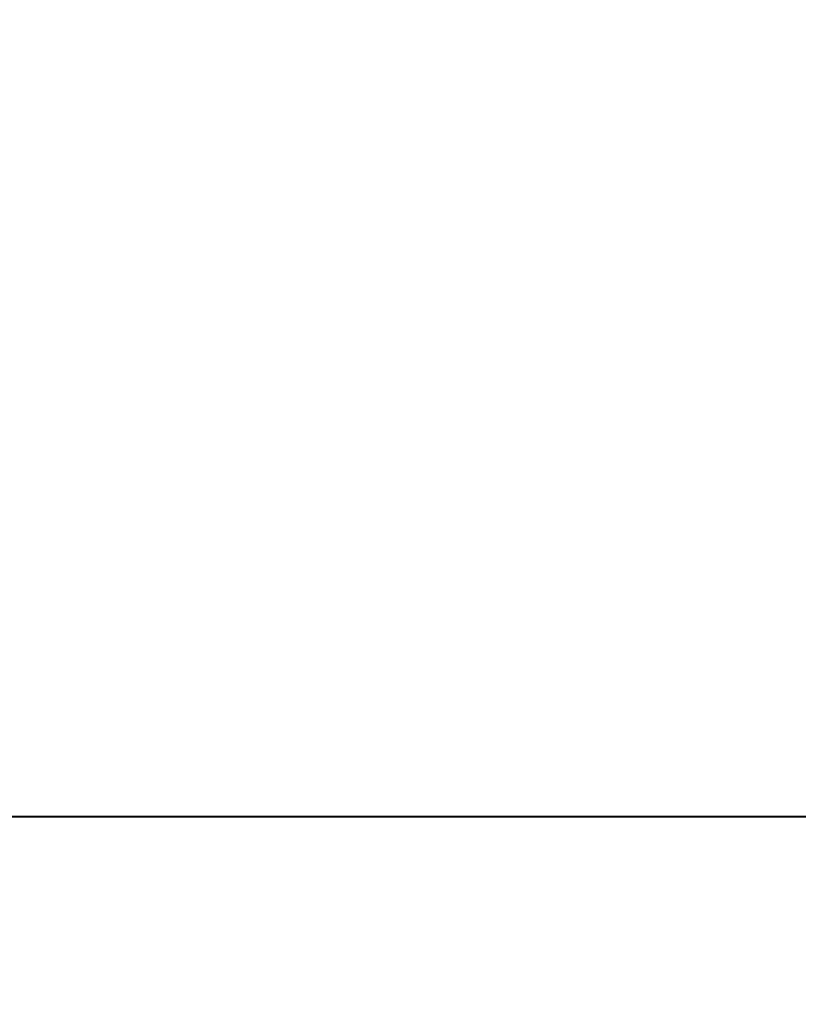
# Model space of a CAD drawing. Units: inches. Extents: x 459864 to 460310, y 324185 to 324787.
# Tile 80 of 112: x 460238.11 to 460246.61, y 324281.44 to 324292.19. Entities that reach past the tile are written whole.
import ezdxf

# ---------------------------------------------------------------- set-up
doc = ezdxf.new("R2010")
doc.units = ezdxf.units.IN
for name, color, linetype, lineweight in [('A-ANNO-DIMS', 2, 'Continuous', 18), ('A-WALL', 7, 'Continuous', 40), ('L-SITE-PATT', 252, 'Continuous', 13)]:
    doc.layers.add(name, color=color, linetype=linetype, lineweight=lineweight)
doc.styles.get("Standard").update_dxf_attribs({"font": 'arial.ttf'})
doc.dimstyles.new('ISO-25', dxfattribs={"dimtxt": 6, "dimasz": 2.5, "dimexe": 1.25, "dimexo": 0.625, "dimtad": 1, "dimdec": 1, "dimlunit": 3, "dimtxsty": 'Standard', "dimcen": 2.5, "dimadec": 0, "dimazin": 0, "dimtfac": 1, "dimtdec": 1, "dimtmove": 0, "dimatfit": 3, "dimfxl": 1, "dimarcsym": 0})

# ---------------------------------------------------------------- blocks, each defined once
blk = doc.blocks.new('*D67')
at = {"layer": 'A-ANNO-DIMS', "color": 0, "lineweight": -2, "transparency": 16777216}
for p, q in [((460208.115, 324284.108), (460208.115, 324315.133)), ((460247.115, 324284.108), (460247.115, 324315.133)), ((460210.615, 324313.883), (460244.615, 324313.883))]:
    blk.add_line(p, q, dxfattribs=at)
at = {"layer": 'A-ANNO-DIMS', "color": 0, "transparency": 16777216}
for points in [[(460210.615, 324314.3), (460210.615, 324313.467), (460208.115, 324313.883)], [(460244.615, 324314.3), (460244.615, 324313.467), (460247.115, 324313.883)]]:
    blk.add_solid(points, dxfattribs=at)
at = {"layer": 'Defpoints', "color": 0, "transparency": 16777216}
for p in [(460247.115, 324313.883), (460208.115, 324283.483), (460247.115, 324283.483)]:
    blk.add_point(p, dxfattribs=at)
at = {"layer": 'A-ANNO-DIMS', "color": 0, "transparency": 16777216, "insert": (460227.615, 324317.574), "char_height": 6, "attachment_point": 5}
blk.add_mtext('3\'-3"', dxfattribs=at)

msp = doc.modelspace()

# ---------------------------------------------------------------- hatches: boundary and pattern name
at = {"layer": 'L-SITE-PATT'}
h = msp.add_hatch(dxfattribs=at)
h.set_pattern_fill('DOTS', color=256)
h.paths.add_polyline_path([(460269.804, 324283.483), (460247.115, 324283.483), (460121.929, 324283.483), (460121.929, 324252.473), (460117.429, 324252.473), (460110.124, 324252.473), (460110.124, 324243.287), (460080.83, 324243.287), (460080.83, 324252.473), (460061.115, 324252.473), (460061.115, 324251.882), (460077.909, 324251.882), (460077.909, 324199.483), (460080.83, 324199.483), (460080.83, 324207.553), (460110.124, 324207.553), (460110.124, 324199.483), (460110.813, 324199.483), (460262.115, 324199.483), (460269.804, 324199.483)], flags=17)
edge = h.paths.add_edge_path(flags=0)
edge.add_ellipse((460222.59, 324263.813), major_axis=(-8.485, 8.485), ratio=1, start_angle=405, end_angle=495, ccw=False)
edge.add_line((460214.821, 324254.66), (460214.832, 324254.666))
edge.add_ellipse((460222.59, 324263.813), major_axis=(-8.485, 8.485), ratio=1, start_angle=405, end_angle=495, ccw=False)
edge.add_line((460210.759, 324261.781), (460210.768, 324261.787))
edge.add_ellipse((460222.59, 324263.813), major_axis=(-8.485, 8.485), ratio=1, start_angle=405, end_angle=495, ccw=False)
edge.add_ellipse((460222.59, 324263.813), major_axis=(-8.485, 8.485), ratio=1, start_angle=392.754, end_angle=405, ccw=False)
edge.add_ellipse((460222.59, 324263.813), major_axis=(-8.485, 8.485), ratio=1, start_angle=380.9347, end_angle=392.754, ccw=False)
edge.add_line((460211.337, 324267.985), (460211.34, 324267.985))
edge.add_ellipse((460222.59, 324263.813), major_axis=(-8.485, 8.485), ratio=1, start_angle=380.9347, end_angle=392.754, ccw=False)
edge.add_ellipse((460222.59, 324263.813), major_axis=(-8.485, 8.485), ratio=1, start_angle=347.9015, end_angle=380.9347, ccw=False)
edge.add_ellipse((460222.59, 324263.813), major_axis=(-8.485, 8.485), ratio=1, start_angle=327.0619, end_angle=347.9015, ccw=False)
edge.add_ellipse((460222.59, 324263.813), major_axis=(-8.485, 8.485), ratio=1, start_angle=278.3246, end_angle=327.0619, ccw=False)
edge.add_line((460225.158, 324275.536), (460225.158, 324275.535))
edge.add_ellipse((460222.59, 324263.813), major_axis=(-8.485, 8.485), ratio=1, start_angle=278.3246, end_angle=327.0619, ccw=False)
edge.add_ellipse((460222.59, 324263.813), major_axis=(-8.485, 8.485), ratio=1, start_angle=260.6436, end_angle=278.3246, ccw=False)
edge.add_ellipse((460222.59, 324263.813), major_axis=(-8.485, 8.485), ratio=1, start_angle=225, end_angle=260.6436, ccw=False)
edge.add_line((460234.509, 324265.243), (460234.501, 324265.239))
edge.add_ellipse((460222.59, 324263.813), major_axis=(-8.485, 8.485), ratio=1, start_angle=225, end_angle=260.6436, ccw=False)
edge.add_ellipse((460222.59, 324263.813), major_axis=(-8.485, 8.485), ratio=1, start_angle=495, end_angle=585, ccw=False)
edge.add_line((460234.437, 324261.861), (460234.424, 324261.858))
edge.add_ellipse((460222.59, 324263.813), major_axis=(-8.485, 8.485), ratio=1, start_angle=495, end_angle=585, ccw=False)
edge.add_line((460227.95, 324253.067), (460227.946, 324253.083))
edge.add_ellipse((460222.59, 324263.813), major_axis=(-8.485, 8.485), ratio=1, start_angle=495, end_angle=585, ccw=False)
edge.add_line((460226.223, 324252.369), (460226.211, 324252.38))
edge.add_ellipse((460222.59, 324263.813), major_axis=(-8.485, 8.485), ratio=1, start_angle=495, end_angle=585, ccw=False)
h.paths.add_polyline_path([(460219.651, 324254.347), (460218.461, 324253.545), (460218.275, 324254.789), (460219.642, 324256.542), (460219.625, 324260.848), (460216.11, 324257.333), (460214.35, 324256.978), (460215.416, 324259.356), (460212.524, 324258.496), (460213.137, 324259.93), (460218.507, 324263.813), (460222.59, 324263.813), (460222.59, 324267.807), (460218.176, 324272.212), (460219.026, 324274.639), (460222.59, 324272.811), (460222.59, 324275.423), (460223.057, 324274.825), (460222.675, 324273.492), (460225.912, 324267.135), (460219.625, 324260.848)], flags=0)
edge = h.paths.add_edge_path(flags=0)
edge.add_ellipse((460194.576, 324264.046), major_axis=(-8.485, 8.485), ratio=1, start_angle=495, end_angle=585, ccw=False)
edge.add_line((460199.936, 324253.3), (460199.932, 324253.316))
edge.add_ellipse((460194.576, 324264.046), major_axis=(-8.485, 8.485), ratio=1, start_angle=495, end_angle=585, ccw=False)
edge.add_line((460198.208, 324252.603), (460198.196, 324252.613))
edge.add_ellipse((460194.576, 324264.046), major_axis=(-8.485, 8.485), ratio=1, start_angle=495, end_angle=585, ccw=False)
edge.add_ellipse((460194.576, 324264.046), major_axis=(-8.485, 8.485), ratio=1, start_angle=405, end_angle=495, ccw=False)
edge.add_line((460186.806, 324254.893), (460186.817, 324254.899))
edge.add_ellipse((460194.576, 324264.046), major_axis=(-8.485, 8.485), ratio=1, start_angle=405, end_angle=495, ccw=False)
edge.add_line((460182.744, 324262.014), (460182.753, 324262.02))
edge.add_ellipse((460194.576, 324264.046), major_axis=(-8.485, 8.485), ratio=1, start_angle=405, end_angle=495, ccw=False)
edge.add_ellipse((460194.576, 324264.046), major_axis=(-8.485, 8.485), ratio=1, start_angle=392.754, end_angle=405, ccw=False)
edge.add_ellipse((460194.576, 324264.046), major_axis=(-8.485, 8.485), ratio=1, start_angle=380.9347, end_angle=392.754, ccw=False)
edge.add_line((460183.323, 324268.218), (460183.326, 324268.218))
edge.add_ellipse((460194.576, 324264.046), major_axis=(-8.485, 8.485), ratio=1, start_angle=380.9347, end_angle=392.754, ccw=False)
edge.add_ellipse((460194.576, 324264.046), major_axis=(-8.485, 8.485), ratio=1, start_angle=347.9015, end_angle=380.9347, ccw=False)
edge.add_ellipse((460194.576, 324264.046), major_axis=(-8.485, 8.485), ratio=1, start_angle=327.0619, end_angle=347.9015, ccw=False)
edge.add_ellipse((460194.576, 324264.046), major_axis=(-8.485, 8.485), ratio=1, start_angle=278.3246, end_angle=327.0619, ccw=False)
edge.add_line((460197.144, 324275.769), (460197.143, 324275.768))
edge.add_ellipse((460194.576, 324264.046), major_axis=(-8.485, 8.485), ratio=1, start_angle=278.3246, end_angle=327.0619, ccw=False)
edge.add_ellipse((460194.576, 324264.046), major_axis=(-8.485, 8.485), ratio=1, start_angle=260.6436, end_angle=278.3246, ccw=False)
edge.add_ellipse((460194.576, 324264.046), major_axis=(-8.485, 8.485), ratio=1, start_angle=225, end_angle=260.6436, ccw=False)
edge.add_line((460206.494, 324265.476), (460206.487, 324265.473))
edge.add_ellipse((460194.576, 324264.046), major_axis=(-8.485, 8.485), ratio=1, start_angle=225, end_angle=260.6436, ccw=False)
edge.add_ellipse((460194.576, 324264.046), major_axis=(-8.485, 8.485), ratio=1, start_angle=495, end_angle=585, ccw=False)
edge.add_line((460206.422, 324262.094), (460206.409, 324262.091))
h.paths.add_polyline_path([(460191.61, 324261.081), (460191.637, 324254.58), (460190.447, 324253.778), (460190.261, 324255.023), (460191.628, 324256.775), (460191.61, 324261.081), (460188.096, 324257.566), (460186.335, 324257.211), (460187.402, 324259.589), (460184.509, 324258.729), (460185.123, 324260.163), (460190.493, 324264.046), (460194.576, 324264.046), (460194.576, 324268.04), (460190.161, 324272.446), (460191.011, 324274.872), (460194.576, 324273.044), (460194.576, 324275.657), (460195.043, 324275.058), (460194.661, 324273.725), (460197.897, 324267.368)], flags=0)
edge = h.paths.add_edge_path(flags=0)
edge.add_ellipse((460252.912, 324263.578), major_axis=(-8.485, 8.485), ratio=1, start_angle=405, end_angle=495, ccw=False)
edge.add_line((460241.081, 324261.545), (460241.089, 324261.551))
edge.add_ellipse((460252.912, 324263.578), major_axis=(-8.485, 8.485), ratio=1, start_angle=405, end_angle=495, ccw=False)
edge.add_ellipse((460252.912, 324263.578), major_axis=(-8.485, 8.485), ratio=1, start_angle=392.754, end_angle=405, ccw=False)
edge.add_ellipse((460252.912, 324263.578), major_axis=(-8.485, 8.485), ratio=1, start_angle=380.9347, end_angle=392.754, ccw=False)
edge.add_line((460241.659, 324267.749), (460241.662, 324267.749))
edge.add_ellipse((460252.912, 324263.578), major_axis=(-8.485, 8.485), ratio=1, start_angle=380.9347, end_angle=392.754, ccw=False)
edge.add_ellipse((460252.912, 324263.578), major_axis=(-8.485, 8.485), ratio=1, start_angle=347.9015, end_angle=380.9347, ccw=False)
edge.add_ellipse((460252.912, 324263.578), major_axis=(-8.485, 8.485), ratio=1, start_angle=327.0619, end_angle=347.9015, ccw=False)
edge.add_ellipse((460252.912, 324263.578), major_axis=(-8.485, 8.485), ratio=1, start_angle=278.3246, end_angle=327.0619, ccw=False)
edge.add_line((460255.48, 324275.3), (460255.479, 324275.299))
edge.add_ellipse((460252.912, 324263.578), major_axis=(-8.485, 8.485), ratio=1, start_angle=278.3246, end_angle=327.0619, ccw=False)
edge.add_ellipse((460252.912, 324263.578), major_axis=(-8.485, 8.485), ratio=1, start_angle=260.6436, end_angle=278.3246, ccw=False)
edge.add_ellipse((460252.912, 324263.578), major_axis=(-8.485, 8.485), ratio=1, start_angle=225, end_angle=260.6436, ccw=False)
edge.add_line((460264.83, 324265.007), (460264.823, 324265.004))
edge.add_ellipse((460252.912, 324263.578), major_axis=(-8.485, 8.485), ratio=1, start_angle=225, end_angle=260.6436, ccw=False)
edge.add_ellipse((460252.912, 324263.578), major_axis=(-8.485, 8.485), ratio=1, start_angle=495, end_angle=585, ccw=False)
edge.add_line((460264.758, 324261.626), (460264.745, 324261.622))
edge.add_ellipse((460252.912, 324263.578), major_axis=(-8.485, 8.485), ratio=1, start_angle=495, end_angle=585, ccw=False)
edge.add_line((460258.272, 324252.832), (460258.268, 324252.848))
edge.add_ellipse((460252.912, 324263.578), major_axis=(-8.485, 8.485), ratio=1, start_angle=495, end_angle=585, ccw=False)
edge.add_line((460256.545, 324252.134), (460256.533, 324252.144))
edge.add_ellipse((460252.912, 324263.578), major_axis=(-8.485, 8.485), ratio=1, start_angle=495, end_angle=585, ccw=False)
edge.add_ellipse((460252.912, 324263.578), major_axis=(-8.485, 8.485), ratio=1, start_angle=405, end_angle=495, ccw=False)
edge.add_line((460245.143, 324254.424), (460245.153, 324254.43))
h.paths.add_polyline_path([(460244.672, 324256.742), (460245.738, 324259.12), (460242.846, 324258.26), (460243.459, 324259.694), (460248.829, 324263.578), (460252.912, 324263.578), (460252.912, 324267.571), (460248.497, 324271.977), (460249.348, 324274.403), (460252.912, 324272.576), (460252.912, 324275.188), (460253.379, 324274.589), (460252.997, 324273.257), (460256.233, 324266.899), (460249.946, 324260.612), (460249.973, 324254.111), (460248.783, 324253.309), (460248.597, 324254.554), (460249.964, 324256.306), (460249.946, 324260.612), (460246.432, 324257.097)], flags=0)
edge = h.paths.add_edge_path(flags=0)
edge.add_ellipse((460167.439, 324262.833), major_axis=(-8.485, 8.485), ratio=1, start_angle=495, end_angle=585, ccw=False)
edge.add_line((460172.799, 324252.087), (460172.795, 324252.103))
edge.add_ellipse((460167.439, 324262.833), major_axis=(-8.485, 8.485), ratio=1, start_angle=495, end_angle=585, ccw=False)
edge.add_line((460171.071, 324251.389), (460171.059, 324251.399))
edge.add_ellipse((460167.439, 324262.833), major_axis=(-8.485, 8.485), ratio=1, start_angle=495, end_angle=585, ccw=False)
edge.add_ellipse((460167.439, 324262.833), major_axis=(-8.485, 8.485), ratio=1, start_angle=405, end_angle=495, ccw=False)
edge.add_line((460159.669, 324253.679), (460159.68, 324253.685))
edge.add_ellipse((460167.439, 324262.833), major_axis=(-8.485, 8.485), ratio=1, start_angle=405, end_angle=495, ccw=False)
edge.add_line((460155.607, 324260.8), (460155.616, 324260.806))
edge.add_ellipse((460167.439, 324262.833), major_axis=(-8.485, 8.485), ratio=1, start_angle=405, end_angle=495, ccw=False)
edge.add_ellipse((460167.439, 324262.833), major_axis=(-8.485, 8.485), ratio=1, start_angle=392.754, end_angle=405, ccw=False)
edge.add_ellipse((460167.439, 324262.833), major_axis=(-8.485, 8.485), ratio=1, start_angle=380.9347, end_angle=392.754, ccw=False)
edge.add_line((460156.185, 324267.005), (460156.189, 324267.005))
edge.add_ellipse((460167.439, 324262.833), major_axis=(-8.485, 8.485), ratio=1, start_angle=380.9347, end_angle=392.754, ccw=False)
edge.add_ellipse((460167.439, 324262.833), major_axis=(-8.485, 8.485), ratio=1, start_angle=347.9015, end_angle=380.9347, ccw=False)
edge.add_ellipse((460167.439, 324262.833), major_axis=(-8.485, 8.485), ratio=1, start_angle=327.0619, end_angle=347.9015, ccw=False)
edge.add_ellipse((460167.439, 324262.833), major_axis=(-8.485, 8.485), ratio=1, start_angle=278.3246, end_angle=327.0619, ccw=False)
edge.add_line((460170.007, 324274.556), (460170.006, 324274.554))
edge.add_ellipse((460167.439, 324262.833), major_axis=(-8.485, 8.485), ratio=1, start_angle=278.3246, end_angle=327.0619, ccw=False)
edge.add_ellipse((460167.439, 324262.833), major_axis=(-8.485, 8.485), ratio=1, start_angle=260.6436, end_angle=278.3246, ccw=False)
edge.add_ellipse((460167.439, 324262.833), major_axis=(-8.485, 8.485), ratio=1, start_angle=225, end_angle=260.6436, ccw=False)
edge.add_line((460179.357, 324264.262), (460179.35, 324264.259))
edge.add_ellipse((460167.439, 324262.833), major_axis=(-8.485, 8.485), ratio=1, start_angle=225, end_angle=260.6436, ccw=False)
edge.add_ellipse((460167.439, 324262.833), major_axis=(-8.485, 8.485), ratio=1, start_angle=495, end_angle=585, ccw=False)
edge.add_line((460179.285, 324260.881), (460179.272, 324260.877))
h.paths.add_polyline_path([(460164.473, 324259.867), (460164.5, 324253.366), (460163.31, 324252.565), (460163.124, 324253.809), (460164.491, 324255.561), (460164.473, 324259.867), (460160.958, 324256.353), (460159.198, 324255.998), (460160.265, 324258.375), (460157.372, 324257.515), (460157.986, 324258.949), (460163.356, 324262.833), (460167.439, 324262.833), (460167.439, 324266.826), (460163.024, 324271.232), (460163.874, 324273.659), (460167.439, 324271.831), (460167.439, 324274.443), (460167.905, 324273.844), (460167.524, 324272.512), (460170.76, 324266.154)], flags=0)
edge = h.paths.add_edge_path(flags=0)
edge.add_ellipse((460140.758, 324262.37), major_axis=(-8.485, 8.485), ratio=1, start_angle=495, end_angle=585, ccw=False)
edge.add_line((460146.118, 324251.624), (460146.114, 324251.639))
edge.add_ellipse((460140.758, 324262.37), major_axis=(-8.485, 8.485), ratio=1, start_angle=495, end_angle=585, ccw=False)
edge.add_line((460144.391, 324250.926), (460144.379, 324250.936))
edge.add_ellipse((460140.758, 324262.37), major_axis=(-8.485, 8.485), ratio=1, start_angle=495, end_angle=585, ccw=False)
edge.add_ellipse((460140.758, 324262.37), major_axis=(-8.485, 8.485), ratio=1, start_angle=405, end_angle=495, ccw=False)
edge.add_line((460132.989, 324253.216), (460132.999, 324253.222))
edge.add_ellipse((460140.758, 324262.37), major_axis=(-8.485, 8.485), ratio=1, start_angle=405, end_angle=495, ccw=False)
edge.add_line((460128.927, 324260.337), (460128.935, 324260.343))
edge.add_ellipse((460140.758, 324262.37), major_axis=(-8.485, 8.485), ratio=1, start_angle=405, end_angle=495, ccw=False)
edge.add_ellipse((460140.758, 324262.37), major_axis=(-8.485, 8.485), ratio=1, start_angle=392.754, end_angle=405, ccw=False)
edge.add_ellipse((460140.758, 324262.37), major_axis=(-8.485, 8.485), ratio=1, start_angle=380.9347, end_angle=392.754, ccw=False)
edge.add_line((460129.505, 324266.541), (460129.508, 324266.541))
edge.add_ellipse((460140.758, 324262.37), major_axis=(-8.485, 8.485), ratio=1, start_angle=380.9347, end_angle=392.754, ccw=False)
edge.add_ellipse((460140.758, 324262.37), major_axis=(-8.485, 8.485), ratio=1, start_angle=347.9015, end_angle=380.9347, ccw=False)
edge.add_ellipse((460140.758, 324262.37), major_axis=(-8.485, 8.485), ratio=1, start_angle=327.0619, end_angle=347.9015, ccw=False)
edge.add_ellipse((460140.758, 324262.37), major_axis=(-8.485, 8.485), ratio=1, start_angle=278.3246, end_angle=327.0619, ccw=False)
edge.add_line((460143.326, 324274.092), (460143.325, 324274.091))
edge.add_ellipse((460140.758, 324262.37), major_axis=(-8.485, 8.485), ratio=1, start_angle=278.3246, end_angle=327.0619, ccw=False)
edge.add_ellipse((460140.758, 324262.37), major_axis=(-8.485, 8.485), ratio=1, start_angle=260.6436, end_angle=278.3246, ccw=False)
edge.add_ellipse((460140.758, 324262.37), major_axis=(-8.485, 8.485), ratio=1, start_angle=225, end_angle=260.6436, ccw=False)
edge.add_line((460152.677, 324263.799), (460152.669, 324263.796))
edge.add_ellipse((460140.758, 324262.37), major_axis=(-8.485, 8.485), ratio=1, start_angle=225, end_angle=260.6436, ccw=False)
edge.add_ellipse((460140.758, 324262.37), major_axis=(-8.485, 8.485), ratio=1, start_angle=495, end_angle=585, ccw=False)
edge.add_line((460152.604, 324260.418), (460152.592, 324260.414))
h.paths.add_polyline_path([(460137.792, 324259.404), (460137.819, 324252.903), (460136.629, 324252.101), (460136.443, 324253.346), (460137.81, 324255.098), (460137.792, 324259.404), (460134.278, 324255.889), (460132.518, 324255.534), (460133.584, 324257.912), (460130.692, 324257.052), (460131.305, 324258.486), (460136.675, 324262.37), (460140.758, 324262.37), (460140.758, 324266.363), (460136.343, 324270.769), (460137.194, 324273.195), (460140.758, 324271.367), (460140.758, 324273.98), (460141.225, 324273.381), (460140.843, 324272.049), (460144.079, 324265.691)], flags=0)
h.paths.add_polyline_path([(460110.124, 324227.414), (460080.83, 324227.414), (460080.83, 324235.484), (460110.124, 324235.484)], flags=16)
h.paths.add_polyline_path([(460110.124, 324220.797), (460110.124, 324212.727), (460080.83, 324212.727), (460080.83, 324220.797)], flags=16)
h.paths.add_polyline_path([(460269.804, 324283.483), (460247.115, 324283.483), (460121.929, 324283.483), (460121.929, 324252.473), (460117.429, 324252.473), (460110.124, 324252.473), (460110.124, 324243.287), (460080.83, 324243.287), (460080.83, 324252.473), (460061.115, 324252.473), (460061.115, 324251.882), (460077.909, 324251.882), (460077.909, 324199.483), (460080.83, 324199.483), (460080.83, 324207.553), (460110.124, 324207.553), (460110.124, 324199.483), (460262.115, 324199.483), (460269.804, 324199.483)], flags=17)
h.paths.add_polyline_path([(460219.651, 324254.347), (460218.461, 324253.545), (460218.275, 324254.789), (460219.642, 324256.542), (460219.625, 324260.848), (460216.11, 324257.333), (460214.35, 324256.978), (460215.416, 324259.356), (460212.524, 324258.496), (460213.137, 324259.93), (460218.507, 324263.813), (460222.59, 324263.813), (460220.18, 324266.223), (460215.461, 324265.308), (460211.835, 324266.137), (460216.247, 324267.985), (460218.418, 324267.985), (460222.59, 324263.813), (460222.59, 324267.807), (460218.176, 324272.212), (460219.026, 324274.639), (460222.59, 324272.811), (460222.59, 324275.423), (460223.057, 324274.825), (460222.675, 324273.492), (460225.912, 324267.135), (460222.59, 324263.813), (460231.383, 324263.813), (460228.485, 324262.488), (460224.425, 324261.978), (460228.68, 324257.724), (460228.966, 324254.791), (460227.142, 324256.537), (460227.542, 324254.819), (460227.333, 324253.614), (460222.59, 324259.985), (460222.59, 324255.497), (460221.377, 324256.541), (460220.576, 324261.799), (460219.625, 324260.848)], flags=0)
h.paths.add_polyline_path([(460199.127, 324256.77), (460199.528, 324255.052), (460199.319, 324253.848), (460194.576, 324260.218), (460194.576, 324255.73), (460193.363, 324256.774), (460192.561, 324262.032), (460191.61, 324261.081), (460191.637, 324254.58), (460190.447, 324253.778), (460190.261, 324255.023), (460191.628, 324256.775), (460191.61, 324261.081), (460188.096, 324257.566), (460186.335, 324257.211), (460187.402, 324259.589), (460184.509, 324258.729), (460185.123, 324260.163), (460190.493, 324264.046), (460194.576, 324264.046), (460192.166, 324266.456), (460187.446, 324265.541), (460183.82, 324266.37), (460188.232, 324268.218), (460190.404, 324268.218), (460194.576, 324264.046), (460194.576, 324268.04), (460190.161, 324272.446), (460191.011, 324274.872), (460194.576, 324273.044), (460194.576, 324275.657), (460195.043, 324275.058), (460194.661, 324273.725), (460197.897, 324267.368), (460194.576, 324264.046), (460203.368, 324264.046), (460200.47, 324262.721), (460196.411, 324262.212), (460200.665, 324257.957), (460200.951, 324255.024)], flags=0)
h.paths.add_polyline_path([(460244.672, 324256.742), (460245.738, 324259.12), (460242.846, 324258.26), (460243.459, 324259.694), (460248.829, 324263.578), (460252.912, 324263.578), (460250.502, 324265.987), (460245.783, 324265.072), (460242.156, 324265.901), (460246.568, 324267.749), (460248.74, 324267.749), (460252.912, 324263.578), (460252.912, 324267.571), (460248.497, 324271.977), (460249.348, 324274.403), (460252.912, 324272.576), (460252.912, 324275.188), (460253.379, 324274.589), (460252.997, 324273.257), (460256.233, 324266.899), (460252.912, 324263.578), (460261.705, 324263.578), (460258.806, 324262.252), (460254.747, 324261.743), (460259.002, 324257.488), (460259.288, 324254.555), (460257.463, 324256.301), (460257.864, 324254.583), (460257.655, 324253.379), (460252.912, 324259.749), (460252.912, 324255.261), (460251.699, 324256.305), (460250.897, 324261.563), (460249.946, 324260.612), (460249.973, 324254.111), (460248.783, 324253.309), (460248.597, 324254.554), (460249.964, 324256.306), (460249.946, 324260.612), (460246.432, 324257.097)], flags=0)
h.paths.add_polyline_path([(460173.528, 324256.743), (460173.814, 324253.811), (460171.99, 324255.556), (460172.39, 324253.838), (460172.182, 324252.634), (460167.439, 324259.004), (460167.439, 324254.516), (460166.226, 324255.56), (460165.424, 324260.818), (460164.473, 324259.867), (460164.5, 324253.366), (460163.31, 324252.565), (460163.124, 324253.809), (460164.491, 324255.561), (460164.473, 324259.867), (460160.958, 324256.353), (460159.198, 324255.998), (460160.265, 324258.375), (460157.372, 324257.515), (460157.986, 324258.949), (460163.356, 324262.833), (460167.439, 324262.833), (460165.029, 324265.243), (460160.309, 324264.327), (460156.683, 324265.156), (460161.095, 324267.005), (460163.267, 324267.005), (460167.439, 324262.833), (460167.439, 324266.826), (460163.024, 324271.232), (460163.874, 324273.659), (460167.439, 324271.831), (460167.439, 324274.443), (460167.905, 324273.844), (460167.524, 324272.512), (460170.76, 324266.154), (460167.439, 324262.833), (460176.231, 324262.833), (460173.333, 324261.507), (460169.274, 324260.998)], flags=0)
h.paths.add_polyline_path([(460146.848, 324256.28), (460147.134, 324253.347), (460145.31, 324255.093), (460145.71, 324253.375), (460145.501, 324252.171), (460140.758, 324258.541), (460140.758, 324254.053), (460139.545, 324255.097), (460138.744, 324260.355), (460137.792, 324259.404), (460137.819, 324252.903), (460136.629, 324252.101), (460136.443, 324253.346), (460137.81, 324255.098), (460137.792, 324259.404), (460134.278, 324255.889), (460132.518, 324255.534), (460133.584, 324257.912), (460130.692, 324257.052), (460131.305, 324258.486), (460136.675, 324262.37), (460140.758, 324262.37), (460138.348, 324264.779), (460133.629, 324263.864), (460130.002, 324264.693), (460134.414, 324266.541), (460136.586, 324266.541), (460140.758, 324262.37), (460140.758, 324266.363), (460136.343, 324270.769), (460137.194, 324273.195), (460140.758, 324271.367), (460140.758, 324273.98), (460141.225, 324273.381), (460140.843, 324272.049), (460144.079, 324265.691), (460140.758, 324262.37), (460149.551, 324262.37), (460146.653, 324261.044), (460142.593, 324260.535)], flags=0)
edge = h.paths.add_edge_path()
edge.add_line((460269.804, 324272.549), (460260.881, 324272.549))
edge.add_ellipse((460252.912, 324263.578), major_axis=(-8.485, 8.485), ratio=1, start_angle=260.6436, end_angle=273.3846, ccw=False)
edge.add_line((460262.283, 324271.092), (460262.261, 324271.091))
edge.add_ellipse((460252.912, 324263.578), major_axis=(-8.485, 8.485), ratio=1, start_angle=260.6436, end_angle=273.3846, ccw=False)
edge.add_ellipse((460252.912, 324263.578), major_axis=(-8.485, 8.485), ratio=1, start_angle=225, end_angle=260.6436, ccw=False)
edge.add_line((460263.609, 324269.063), (460263.572, 324269.058))
edge.add_ellipse((460252.912, 324263.578), major_axis=(-8.485, 8.485), ratio=1, start_angle=225, end_angle=260.6436, ccw=False)
edge.add_line((460264.615, 324266.306), (460264.585, 324266.305))
edge.add_ellipse((460252.912, 324263.578), major_axis=(-8.485, 8.485), ratio=1, start_angle=225, end_angle=260.6436, ccw=False)
edge.add_line((460264.83, 324265.007), (460264.823, 324265.004))
edge.add_ellipse((460252.912, 324263.578), major_axis=(-8.485, 8.485), ratio=1, start_angle=225, end_angle=260.6436, ccw=False)
edge.add_ellipse((460252.912, 324263.578), major_axis=(-8.485, 8.485), ratio=1, start_angle=495, end_angle=585, ccw=False)
edge.add_line((460264.758, 324261.626), (460264.745, 324261.622))
edge.add_ellipse((460252.912, 324263.578), major_axis=(-8.485, 8.485), ratio=1, start_angle=495, end_angle=585, ccw=False)
edge.add_line((460263.442, 324257.739), (460263.389, 324257.779))
edge.add_ellipse((460252.912, 324263.578), major_axis=(-8.485, 8.485), ratio=1, start_angle=495, end_angle=585, ccw=False)
edge.add_line((460258.128, 324252.744), (460258.102, 324252.779))
edge.add_ellipse((460252.912, 324263.578), major_axis=(-8.485, 8.485), ratio=1, start_angle=495, end_angle=585, ccw=False)
edge.add_line((460256.545, 324252.134), (460256.533, 324252.144))
edge.add_ellipse((460252.912, 324263.578), major_axis=(-8.485, 8.485), ratio=1, start_angle=495, end_angle=585, ccw=False)
edge.add_ellipse((460252.912, 324263.578), major_axis=(-8.485, 8.485), ratio=1, start_angle=405, end_angle=495, ccw=False)
edge.add_line((460250.594, 324251.78), (460250.605, 324251.82))
edge.add_ellipse((460252.912, 324263.578), major_axis=(-8.485, 8.485), ratio=1, start_angle=405, end_angle=495, ccw=False)
edge.add_line((460245.143, 324254.424), (460245.153, 324254.43))
edge.add_ellipse((460252.912, 324263.578), major_axis=(-8.485, 8.485), ratio=1, start_angle=405, end_angle=495, ccw=False)
edge.add_line((460243.525, 324256.059), (460243.56, 324256.091))
edge.add_ellipse((460252.912, 324263.578), major_axis=(-8.485, 8.485), ratio=1, start_angle=405, end_angle=495, ccw=False)
edge.add_line((460241.44, 324259.893), (460241.522, 324259.896))
edge.add_ellipse((460252.912, 324263.578), major_axis=(-8.485, 8.485), ratio=1, start_angle=405, end_angle=495, ccw=False)
edge.add_line((460241.081, 324261.545), (460241.089, 324261.551))
edge.add_ellipse((460252.912, 324263.578), major_axis=(-8.485, 8.485), ratio=1, start_angle=405, end_angle=495, ccw=False)
edge.add_ellipse((460252.912, 324263.578), major_axis=(-8.485, 8.485), ratio=1, start_angle=392.754, end_angle=405, ccw=False)
edge.add_line((460241.05, 324265.438), (460241.063, 324265.443))
edge.add_ellipse((460252.912, 324263.578), major_axis=(-8.485, 8.485), ratio=1, start_angle=392.754, end_angle=405, ccw=False)
edge.add_ellipse((460252.912, 324263.578), major_axis=(-8.485, 8.485), ratio=1, start_angle=380.9347, end_angle=392.754, ccw=False)
edge.add_line((460241.452, 324267.176), (460241.469, 324267.171))
edge.add_ellipse((460252.912, 324263.578), major_axis=(-8.485, 8.485), ratio=1, start_angle=380.9347, end_angle=392.754, ccw=False)
edge.add_line((460241.659, 324267.749), (460241.662, 324267.749))
edge.add_ellipse((460252.912, 324263.578), major_axis=(-8.485, 8.485), ratio=1, start_angle=380.9347, end_angle=392.754, ccw=False)
edge.add_ellipse((460252.912, 324263.578), major_axis=(-8.485, 8.485), ratio=1, start_angle=356.6154, end_angle=380.9347, ccw=False)
edge.add_line((460244.88, 324272.488), (460244.713, 324272.549))
edge.add_line((460244.713, 324272.549), (460230.817, 324272.549))
edge.add_ellipse((460222.59, 324263.813), major_axis=(-8.485, 8.485), ratio=1, start_angle=260.6436, end_angle=271.7178, ccw=False)
edge.add_ellipse((460222.59, 324263.813), major_axis=(-8.485, 8.485), ratio=1, start_angle=225, end_angle=260.6436, ccw=False)
edge.add_line((460233.287, 324269.299), (460233.25, 324269.294))
edge.add_ellipse((460222.59, 324263.813), major_axis=(-8.485, 8.485), ratio=1, start_angle=225, end_angle=260.6436, ccw=False)
edge.add_line((460234.294, 324266.541), (460234.264, 324266.541))
edge.add_ellipse((460222.59, 324263.813), major_axis=(-8.485, 8.485), ratio=1, start_angle=225, end_angle=260.6436, ccw=False)
edge.add_line((460234.509, 324265.243), (460234.501, 324265.239))
edge.add_ellipse((460222.59, 324263.813), major_axis=(-8.485, 8.485), ratio=1, start_angle=225, end_angle=260.6436, ccw=False)
edge.add_ellipse((460222.59, 324263.813), major_axis=(-8.485, 8.485), ratio=1, start_angle=495, end_angle=585, ccw=False)
edge.add_line((460234.437, 324261.861), (460234.424, 324261.858))
edge.add_ellipse((460222.59, 324263.813), major_axis=(-8.485, 8.485), ratio=1, start_angle=495, end_angle=585, ccw=False)
edge.add_line((460233.121, 324257.975), (460233.068, 324258.015))
edge.add_ellipse((460222.59, 324263.813), major_axis=(-8.485, 8.485), ratio=1, start_angle=495, end_angle=585, ccw=False)
edge.add_line((460227.806, 324252.979), (460227.78, 324253.014))
edge.add_ellipse((460222.59, 324263.813), major_axis=(-8.485, 8.485), ratio=1, start_angle=495, end_angle=585, ccw=False)
edge.add_line((460226.223, 324252.369), (460226.211, 324252.38))
edge.add_ellipse((460222.59, 324263.813), major_axis=(-8.485, 8.485), ratio=1, start_angle=495, end_angle=585, ccw=False)
edge.add_ellipse((460222.59, 324263.813), major_axis=(-8.485, 8.485), ratio=1, start_angle=405, end_angle=495, ccw=False)
edge.add_line((460220.272, 324252.016), (460220.283, 324252.055))
edge.add_ellipse((460222.59, 324263.813), major_axis=(-8.485, 8.485), ratio=1, start_angle=405, end_angle=495, ccw=False)
edge.add_line((460214.821, 324254.66), (460214.832, 324254.666))
edge.add_ellipse((460222.59, 324263.813), major_axis=(-8.485, 8.485), ratio=1, start_angle=405, end_angle=495, ccw=False)
edge.add_line((460213.203, 324256.295), (460213.239, 324256.327))
edge.add_ellipse((460222.59, 324263.813), major_axis=(-8.485, 8.485), ratio=1, start_angle=405, end_angle=495, ccw=False)
edge.add_line((460211.118, 324260.128), (460211.201, 324260.131))
edge.add_ellipse((460222.59, 324263.813), major_axis=(-8.485, 8.485), ratio=1, start_angle=405, end_angle=495, ccw=False)
edge.add_line((460210.759, 324261.781), (460210.768, 324261.787))
edge.add_ellipse((460222.59, 324263.813), major_axis=(-8.485, 8.485), ratio=1, start_angle=405, end_angle=495, ccw=False)
edge.add_ellipse((460222.59, 324263.813), major_axis=(-8.485, 8.485), ratio=1, start_angle=392.754, end_angle=405, ccw=False)
edge.add_line((460210.729, 324265.673), (460210.741, 324265.678))
edge.add_ellipse((460222.59, 324263.813), major_axis=(-8.485, 8.485), ratio=1, start_angle=392.754, end_angle=405, ccw=False)
edge.add_ellipse((460222.59, 324263.813), major_axis=(-8.485, 8.485), ratio=1, start_angle=380.9347, end_angle=392.754, ccw=False)
edge.add_line((460211.13, 324267.412), (460211.147, 324267.407))
edge.add_ellipse((460222.59, 324263.813), major_axis=(-8.485, 8.485), ratio=1, start_angle=380.9347, end_angle=392.754, ccw=False)
edge.add_line((460211.337, 324267.985), (460211.34, 324267.985))
edge.add_ellipse((460222.59, 324263.813), major_axis=(-8.485, 8.485), ratio=1, start_angle=380.9347, end_angle=392.754, ccw=False)
edge.add_ellipse((460222.59, 324263.813), major_axis=(-8.485, 8.485), ratio=1, start_angle=358.2822, end_angle=380.9347, ccw=False)
edge.add_line((460213.705, 324271.902), (460213.709, 324271.869))
edge.add_ellipse((460222.59, 324263.813), major_axis=(-8.485, 8.485), ratio=1, start_angle=358.2822, end_angle=380.9347, ccw=False)
edge.add_line((460214.363, 324272.549), (460203.078, 324272.549))
edge.add_line((460203.078, 324272.549), (460203.06, 324272.531))
edge.add_ellipse((460194.576, 324264.046), major_axis=(-8.485, 8.485), ratio=1, start_angle=260.6436, end_angle=270.1168, ccw=False)
edge.add_line((460203.957, 324271.561), (460203.921, 324271.56))
edge.add_ellipse((460194.576, 324264.046), major_axis=(-8.485, 8.485), ratio=1, start_angle=260.6436, end_angle=270.1168, ccw=False)
edge.add_ellipse((460194.576, 324264.046), major_axis=(-8.485, 8.485), ratio=1, start_angle=225, end_angle=260.6436, ccw=False)
edge.add_line((460205.272, 324269.532), (460205.235, 324269.527))
edge.add_ellipse((460194.576, 324264.046), major_axis=(-8.485, 8.485), ratio=1, start_angle=225, end_angle=260.6436, ccw=False)
edge.add_line((460206.279, 324266.774), (460206.249, 324266.774))
edge.add_ellipse((460194.576, 324264.046), major_axis=(-8.485, 8.485), ratio=1, start_angle=225, end_angle=260.6436, ccw=False)
edge.add_line((460206.494, 324265.476), (460206.487, 324265.473))
edge.add_ellipse((460194.576, 324264.046), major_axis=(-8.485, 8.485), ratio=1, start_angle=225, end_angle=260.6436, ccw=False)
edge.add_ellipse((460194.576, 324264.046), major_axis=(-8.485, 8.485), ratio=1, start_angle=495, end_angle=585, ccw=False)
edge.add_line((460206.422, 324262.094), (460206.409, 324262.091))
edge.add_ellipse((460194.576, 324264.046), major_axis=(-8.485, 8.485), ratio=1, start_angle=495, end_angle=585, ccw=False)
edge.add_line((460205.106, 324258.208), (460205.053, 324258.248))
edge.add_ellipse((460194.576, 324264.046), major_axis=(-8.485, 8.485), ratio=1, start_angle=495, end_angle=585, ccw=False)
edge.add_line((460199.792, 324253.212), (460199.766, 324253.248))
edge.add_ellipse((460194.576, 324264.046), major_axis=(-8.485, 8.485), ratio=1, start_angle=495, end_angle=585, ccw=False)
edge.add_line((460198.208, 324252.603), (460198.196, 324252.613))
edge.add_ellipse((460194.576, 324264.046), major_axis=(-8.485, 8.485), ratio=1, start_angle=495, end_angle=585, ccw=False)
edge.add_ellipse((460194.576, 324264.046), major_axis=(-8.485, 8.485), ratio=1, start_angle=405, end_angle=495, ccw=False)
edge.add_line((460192.258, 324252.249), (460192.268, 324252.289))
edge.add_ellipse((460194.576, 324264.046), major_axis=(-8.485, 8.485), ratio=1, start_angle=405, end_angle=495, ccw=False)
edge.add_line((460186.806, 324254.893), (460186.817, 324254.899))
edge.add_ellipse((460194.576, 324264.046), major_axis=(-8.485, 8.485), ratio=1, start_angle=405, end_angle=495, ccw=False)
edge.add_line((460185.188, 324256.528), (460185.224, 324256.56))
edge.add_ellipse((460194.576, 324264.046), major_axis=(-8.485, 8.485), ratio=1, start_angle=405, end_angle=495, ccw=False)
edge.add_line((460183.104, 324260.362), (460183.186, 324260.365))
edge.add_ellipse((460194.576, 324264.046), major_axis=(-8.485, 8.485), ratio=1, start_angle=405, end_angle=495, ccw=False)
edge.add_line((460182.744, 324262.014), (460182.753, 324262.02))
edge.add_ellipse((460194.576, 324264.046), major_axis=(-8.485, 8.485), ratio=1, start_angle=405, end_angle=495, ccw=False)
edge.add_ellipse((460194.576, 324264.046), major_axis=(-8.485, 8.485), ratio=1, start_angle=392.754, end_angle=405, ccw=False)
edge.add_line((460182.714, 324265.906), (460182.726, 324265.912))
edge.add_ellipse((460194.576, 324264.046), major_axis=(-8.485, 8.485), ratio=1, start_angle=392.754, end_angle=405, ccw=False)
edge.add_ellipse((460194.576, 324264.046), major_axis=(-8.485, 8.485), ratio=1, start_angle=380.9347, end_angle=392.754, ccw=False)
edge.add_line((460183.116, 324267.645), (460183.133, 324267.64))
edge.add_ellipse((460194.576, 324264.046), major_axis=(-8.485, 8.485), ratio=1, start_angle=380.9347, end_angle=392.754, ccw=False)
edge.add_line((460183.323, 324268.218), (460183.326, 324268.218))
edge.add_ellipse((460194.576, 324264.046), major_axis=(-8.485, 8.485), ratio=1, start_angle=380.9347, end_angle=392.754, ccw=False)
edge.add_ellipse((460194.576, 324264.046), major_axis=(-8.485, 8.485), ratio=1, start_angle=359.8832, end_angle=380.9347, ccw=False)
edge.add_line((460184.491, 324270.611), (460184.553, 324270.611))
edge.add_ellipse((460194.576, 324264.046), major_axis=(-8.485, 8.485), ratio=1, start_angle=359.8832, end_angle=380.9347, ccw=False)
edge.add_line((460185.346, 324271.76), (460185.379, 324271.728))
edge.add_ellipse((460194.576, 324264.046), major_axis=(-8.485, 8.485), ratio=1, start_angle=359.8832, end_angle=380.9347, ccw=False)
edge.add_line((460185.697, 324272.086), (460185.633, 324272.549))
edge.add_line((460185.633, 324272.549), (460174.683, 324272.549))
edge.add_line((460174.683, 324272.549), (460174.606, 324272.457))
edge.add_ellipse((460167.439, 324262.833), major_axis=(-8.485, 8.485), ratio=1, start_angle=260.6436, end_angle=278.3246, ccw=False)
edge.add_ellipse((460167.439, 324262.833), major_axis=(-8.485, 8.485), ratio=1, start_angle=225, end_angle=260.6436, ccw=False)
edge.add_line((460178.135, 324268.318), (460178.098, 324268.313))
edge.add_ellipse((460167.439, 324262.833), major_axis=(-8.485, 8.485), ratio=1, start_angle=225, end_angle=260.6436, ccw=False)
edge.add_line((460179.142, 324265.561), (460179.112, 324265.56))
edge.add_ellipse((460167.439, 324262.833), major_axis=(-8.485, 8.485), ratio=1, start_angle=225, end_angle=260.6436, ccw=False)
edge.add_line((460179.357, 324264.262), (460179.35, 324264.259))
edge.add_ellipse((460167.439, 324262.833), major_axis=(-8.485, 8.485), ratio=1, start_angle=225, end_angle=260.6436, ccw=False)
edge.add_ellipse((460167.439, 324262.833), major_axis=(-8.485, 8.485), ratio=1, start_angle=495, end_angle=585, ccw=False)
edge.add_line((460179.285, 324260.881), (460179.272, 324260.877))
edge.add_ellipse((460167.439, 324262.833), major_axis=(-8.485, 8.485), ratio=1, start_angle=495, end_angle=585, ccw=False)
edge.add_line((460177.969, 324256.994), (460177.916, 324257.034))
edge.add_ellipse((460167.439, 324262.833), major_axis=(-8.485, 8.485), ratio=1, start_angle=495, end_angle=585, ccw=False)
edge.add_line((460172.655, 324251.999), (460172.629, 324252.034))
edge.add_ellipse((460167.439, 324262.833), major_axis=(-8.485, 8.485), ratio=1, start_angle=495, end_angle=585, ccw=False)
edge.add_line((460171.071, 324251.389), (460171.059, 324251.399))
edge.add_ellipse((460167.439, 324262.833), major_axis=(-8.485, 8.485), ratio=1, start_angle=495, end_angle=585, ccw=False)
edge.add_ellipse((460167.439, 324262.833), major_axis=(-8.485, 8.485), ratio=1, start_angle=405, end_angle=495, ccw=False)
edge.add_line((460165.121, 324251.036), (460165.131, 324251.075))
edge.add_ellipse((460167.439, 324262.833), major_axis=(-8.485, 8.485), ratio=1, start_angle=405, end_angle=495, ccw=False)
edge.add_line((460159.669, 324253.679), (460159.68, 324253.685))
edge.add_ellipse((460167.439, 324262.833), major_axis=(-8.485, 8.485), ratio=1, start_angle=405, end_angle=495, ccw=False)
edge.add_line((460158.051, 324255.314), (460158.087, 324255.347))
edge.add_ellipse((460167.439, 324262.833), major_axis=(-8.485, 8.485), ratio=1, start_angle=405, end_angle=495, ccw=False)
edge.add_line((460155.967, 324259.148), (460156.049, 324259.151))
edge.add_ellipse((460167.439, 324262.833), major_axis=(-8.485, 8.485), ratio=1, start_angle=405, end_angle=495, ccw=False)
edge.add_line((460155.607, 324260.8), (460155.616, 324260.806))
edge.add_ellipse((460167.439, 324262.833), major_axis=(-8.485, 8.485), ratio=1, start_angle=405, end_angle=495, ccw=False)
edge.add_ellipse((460167.439, 324262.833), major_axis=(-8.485, 8.485), ratio=1, start_angle=392.754, end_angle=405, ccw=False)
edge.add_line((460155.577, 324264.693), (460155.589, 324264.698))
edge.add_ellipse((460167.439, 324262.833), major_axis=(-8.485, 8.485), ratio=1, start_angle=392.754, end_angle=405, ccw=False)
edge.add_ellipse((460167.439, 324262.833), major_axis=(-8.485, 8.485), ratio=1, start_angle=380.9347, end_angle=392.754, ccw=False)
edge.add_line((460155.979, 324266.432), (460155.996, 324266.426))
edge.add_ellipse((460167.439, 324262.833), major_axis=(-8.485, 8.485), ratio=1, start_angle=380.9347, end_angle=392.754, ccw=False)
edge.add_line((460156.185, 324267.005), (460156.189, 324267.005))
edge.add_ellipse((460167.439, 324262.833), major_axis=(-8.485, 8.485), ratio=1, start_angle=380.9347, end_angle=392.754, ccw=False)
edge.add_ellipse((460167.439, 324262.833), major_axis=(-8.485, 8.485), ratio=1, start_angle=350.9345, end_angle=380.9347, ccw=False)
edge.add_line((460157.363, 324269.397), (460157.414, 324269.397))
edge.add_ellipse((460167.439, 324262.833), major_axis=(-8.485, 8.485), ratio=1, start_angle=350.9345, end_angle=380.9347, ccw=False)
edge.add_line((460158.221, 324270.535), (460158.236, 324270.519))
edge.add_ellipse((460167.439, 324262.833), major_axis=(-8.485, 8.485), ratio=1, start_angle=350.9345, end_angle=380.9347, ccw=False)
edge.add_line((460159.379, 324271.753), (460159.419, 324271.738))
edge.add_ellipse((460167.439, 324262.833), major_axis=(-8.485, 8.485), ratio=1, start_angle=350.9345, end_angle=380.9347, ccw=False)
edge.add_line((460160.396, 324272.549), (460147.112, 324272.549))
edge.add_ellipse((460140.758, 324262.37), major_axis=(-8.485, 8.485), ratio=1, start_angle=278.3246, end_angle=283.0261, ccw=False)
edge.add_ellipse((460140.758, 324262.37), major_axis=(-8.485, 8.485), ratio=1, start_angle=260.6436, end_angle=278.3246, ccw=False)
edge.add_ellipse((460140.758, 324262.37), major_axis=(-8.485, 8.485), ratio=1, start_angle=225, end_angle=260.6436, ccw=False)
edge.add_line((460151.455, 324267.855), (460151.418, 324267.85))
edge.add_ellipse((460140.758, 324262.37), major_axis=(-8.485, 8.485), ratio=1, start_angle=225, end_angle=260.6436, ccw=False)
edge.add_line((460152.462, 324265.098), (460152.431, 324265.097))
edge.add_ellipse((460140.758, 324262.37), major_axis=(-8.485, 8.485), ratio=1, start_angle=225, end_angle=260.6436, ccw=False)
edge.add_line((460152.677, 324263.799), (460152.669, 324263.796))
edge.add_ellipse((460140.758, 324262.37), major_axis=(-8.485, 8.485), ratio=1, start_angle=225, end_angle=260.6436, ccw=False)
edge.add_ellipse((460140.758, 324262.37), major_axis=(-8.485, 8.485), ratio=1, start_angle=495, end_angle=585, ccw=False)
edge.add_line((460152.604, 324260.418), (460152.592, 324260.414))
edge.add_ellipse((460140.758, 324262.37), major_axis=(-8.485, 8.485), ratio=1, start_angle=495, end_angle=585, ccw=False)
edge.add_line((460151.288, 324256.531), (460151.235, 324256.571))
edge.add_ellipse((460140.758, 324262.37), major_axis=(-8.485, 8.485), ratio=1, start_angle=495, end_angle=585, ccw=False)
edge.add_line((460145.974, 324251.535), (460145.948, 324251.571))
edge.add_ellipse((460140.758, 324262.37), major_axis=(-8.485, 8.485), ratio=1, start_angle=495, end_angle=585, ccw=False)
edge.add_line((460144.391, 324250.926), (460144.379, 324250.936))
edge.add_ellipse((460140.758, 324262.37), major_axis=(-8.485, 8.485), ratio=1, start_angle=495, end_angle=585, ccw=False)
edge.add_ellipse((460140.758, 324262.37), major_axis=(-8.485, 8.485), ratio=1, start_angle=405, end_angle=495, ccw=False)
edge.add_line((460138.44, 324250.572), (460138.451, 324250.612))
edge.add_ellipse((460140.758, 324262.37), major_axis=(-8.485, 8.485), ratio=1, start_angle=405, end_angle=495, ccw=False)
edge.add_line((460132.989, 324253.216), (460132.999, 324253.222))
edge.add_ellipse((460140.758, 324262.37), major_axis=(-8.485, 8.485), ratio=1, start_angle=405, end_angle=495, ccw=False)
edge.add_line((460131.371, 324254.851), (460131.406, 324254.883))
edge.add_ellipse((460140.758, 324262.37), major_axis=(-8.485, 8.485), ratio=1, start_angle=405, end_angle=495, ccw=False)
edge.add_line((460129.286, 324258.685), (460129.369, 324258.688))
edge.add_ellipse((460140.758, 324262.37), major_axis=(-8.485, 8.485), ratio=1, start_angle=405, end_angle=495, ccw=False)
edge.add_line((460128.927, 324260.337), (460128.935, 324260.343))
edge.add_ellipse((460140.758, 324262.37), major_axis=(-8.485, 8.485), ratio=1, start_angle=405, end_angle=495, ccw=False)
edge.add_ellipse((460140.758, 324262.37), major_axis=(-8.485, 8.485), ratio=1, start_angle=392.754, end_angle=405, ccw=False)
edge.add_line((460128.896, 324264.23), (460128.909, 324264.235))
edge.add_ellipse((460140.758, 324262.37), major_axis=(-8.485, 8.485), ratio=1, start_angle=392.754, end_angle=405, ccw=False)
edge.add_ellipse((460140.758, 324262.37), major_axis=(-8.485, 8.485), ratio=1, start_angle=380.9347, end_angle=392.754, ccw=False)
edge.add_line((460129.298, 324265.968), (460129.315, 324265.963))
edge.add_ellipse((460140.758, 324262.37), major_axis=(-8.485, 8.485), ratio=1, start_angle=380.9347, end_angle=392.754, ccw=False)
edge.add_line((460129.505, 324266.541), (460129.508, 324266.541))
edge.add_ellipse((460140.758, 324262.37), major_axis=(-8.485, 8.485), ratio=1, start_angle=380.9347, end_angle=392.754, ccw=False)
edge.add_ellipse((460140.758, 324262.37), major_axis=(-8.485, 8.485), ratio=1, start_angle=347.9015, end_angle=380.9347, ccw=False)
edge.add_line((460130.697, 324268.934), (460130.727, 324268.934))
edge.add_ellipse((460140.758, 324262.37), major_axis=(-8.485, 8.485), ratio=1, start_angle=347.9015, end_angle=380.9347, ccw=False)
edge.add_line((460131.869, 324270.48), (460131.879, 324270.413))
edge.add_ellipse((460140.758, 324262.37), major_axis=(-8.485, 8.485), ratio=1, start_angle=347.9015, end_angle=380.9347, ccw=False)
edge.add_line((460132.734, 324271.277), (460132.705, 324271.287))
edge.add_ellipse((460140.758, 324262.37), major_axis=(-8.485, 8.485), ratio=1, start_angle=347.9015, end_angle=380.9347, ccw=False)
edge.add_line((460134.24, 324272.445), (460134.204, 324272.549))
edge.add_line((460134.204, 324272.549), (460121.929, 324272.549))
edge.add_line((460121.929, 324272.549), (460121.929, 324252.473))
edge.add_line((460121.929, 324252.473), (460117.429, 324252.473))
edge.add_line((460117.429, 324252.473), (460110.124, 324252.473))
edge.add_line((460110.124, 324252.473), (460110.124, 324243.287))
edge.add_line((460110.124, 324243.287), (460080.83, 324243.287))
edge.add_line((460080.83, 324243.287), (460080.83, 324252.473))
edge.add_line((460080.83, 324252.473), (460061.115, 324252.473))
edge.add_line((460061.115, 324252.473), (460061.115, 324251.882))
edge.add_line((460061.115, 324251.882), (460077.909, 324251.882))
edge.add_line((460077.909, 324251.882), (460077.909, 324199.483))
edge.add_line((460077.909, 324199.483), (460080.83, 324199.483))
edge.add_line((460080.83, 324199.483), (460080.83, 324207.553))
edge.add_line((460080.83, 324207.553), (460110.124, 324207.553))
edge.add_line((460110.124, 324207.553), (460110.124, 324199.483))
edge.add_line((460110.124, 324199.483), (460110.813, 324199.483))
edge.add_line((460110.813, 324199.483), (460262.115, 324199.483))
edge.add_line((460262.115, 324199.483), (460269.804, 324199.483))
edge.add_line((460269.804, 324199.483), (460269.804, 324272.549))

# ---------------------------------------------------------------- linework, layer by layer
at = {"layer": 'A-WALL'}
msp.add_line((460247.115, 324283.483), (460061.115, 324283.483), dxfattribs=at)

# ---------------------------------------------------------------- dimensions: what is measured, and where the dimension line sits
at = {"layer": 'A-ANNO-DIMS'}
dim = msp.add_linear_dim(base=(460247.115, 324313.883), p1=(460208.115, 324283.483), p2=(460247.115, 324283.483), dimstyle='ISO-25', override={"dimdec": 1, "dimlfac": 1, "dimrnd": 0, "dimzin": 1, "dimdsep": 46, "dimlunit": 4, "dimfrac": 2}, dxfattribs=at)
dim.commit()
dim.dimension.update_dxf_attribs({"geometry": '*D67', "text_midpoint": (460227.615, 324317.574)})

doc.saveas('drawing.dxf')
